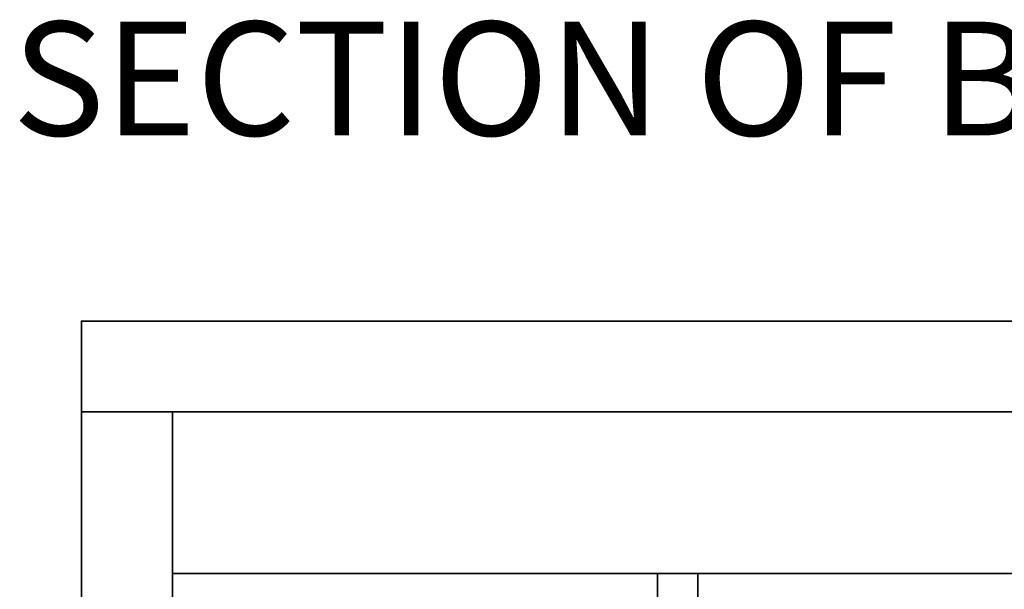
# Model space of a CAD drawing. Units: inches. Extents: x 64 to 1167, y 117 to 939.
# Tile 36 of 56: x 977 to 1074, y 539 to 596. Entities that reach past the tile are written whole.
import ezdxf

# ---------------------------------------------------------------- set-up
doc = ezdxf.new("R2010")
doc.units = ezdxf.units.IN
doc.header["$MEASUREMENT"] = 0
doc.layers.add('A-ANNO-TEXT', color=7, linetype='Continuous', lineweight=25)
doc.layers.add('A-SECT', color=7, linetype='Continuous', lineweight=35)
doc.styles.get("Standard").update_dxf_attribs({"font": 'arial.ttf'})

msp = doc.modelspace()

# ---------------------------------------------------------------- linework, layer by layer
at = {"layer": 'A-SECT'}
for p, q in [((1166.813, 556.679), (982.813, 556.679)), ((991.813, 556.679), (991.813, 436.679)), ((1157.813, 540.679), (991.813, 540.679)), ((1039.813, 540.679), (1039.813, 436.679)), ((1043.813, 540.679), (1043.813, 436.679))]:
    msp.add_line(p, q, dxfattribs=at)
msp.add_lwpolyline([(982.813, 427.679), (1166.813, 427.679), (1166.813, 565.679), (982.813, 565.679)], close=True, dxfattribs=at)

# ---------------------------------------------------------------- texts
at = {"layer": 'A-ANNO-TEXT'}
msp.add_text('SECTION OF BATH ROOM', height=11.26378, dxfattribs=at).set_placement((975.962, 584.046))

doc.saveas('drawing.dxf')
